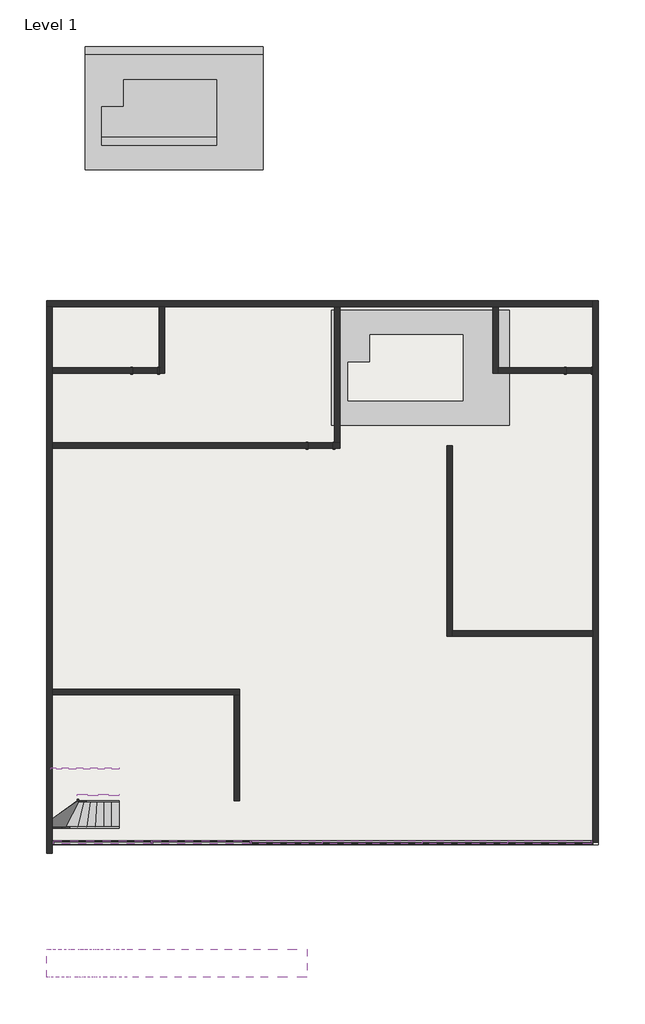
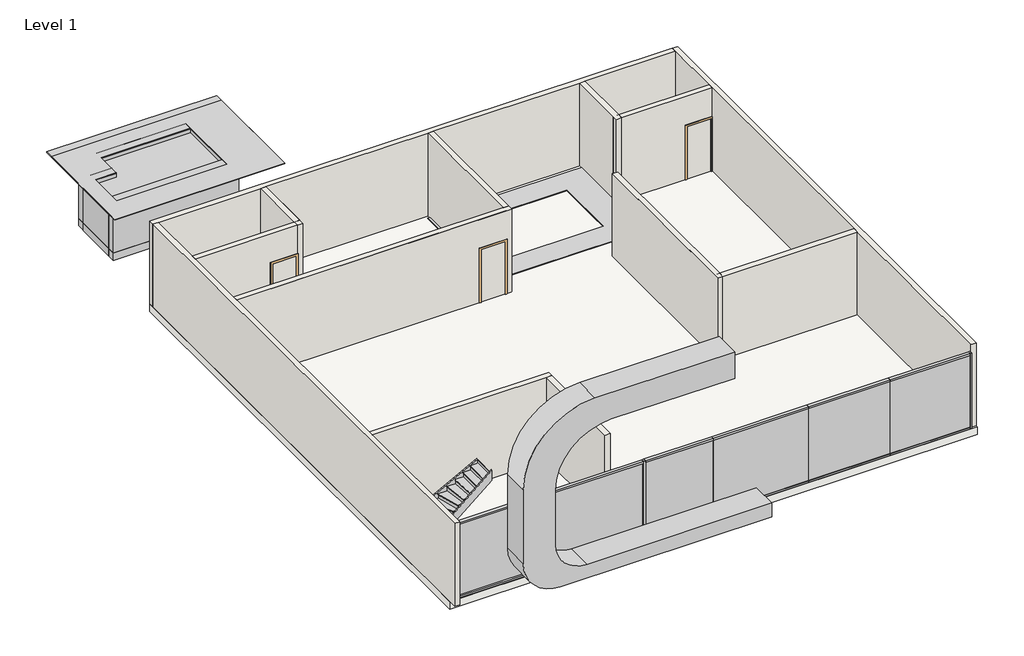
# One storey, incomplete: 32 members, 26 walls, 6 plates, 3 doors, 3 furniture elements, 2 slabs, 2 stair flights, 1 proxy.
"""IFC4 building model written with IfcOpenShell, lengths in millimetres."""

from ifc_helpers import new_model, si_unit, frame, origin, origin_with_axes, place, context, project, spatial, polyline, outline, extrude, faceted_brep, transform, mapped, element, save
from components import generic_models_1_generic_models_1_6508f6ba, door_54dd4da4, door_719f80de, swimming_pool_w_adjustable_terrace_and_size_parametric_16462_e4165495, member_3f395ae9, member_901dee17, member_eaba9652, member_a37e84cf, member_e3dca2c5, member_9f3fc137, member_47c71a51, system_panel_glazed_4ffbc40e, system_panel_glazed_c3829408, system_panel_glazed_34d630f4, system_panel_glazed_dc472efa, system_panel_glazed_7998c3ce, stair_flight_c9f3f3be

model = new_model("IFC4")

# Units and contexts
model_context = context("Model", 3, world=origin())
ifc_project = project(units=[si_unit("LENGTHUNIT", "METRE", prefix="MILLI")], contexts=[model_context])

# Site, building, storey
site = spatial("IfcSite", under=ifc_project)
building = spatial("IfcBuilding", under=site)
storey = spatial("IfcBuildingStorey", under=building, Name="Level 1", Elevation=0.0)

# Proxy
placement = place(None, origin())
generic_models_1_generic_models_1_shape = generic_models_1_generic_models_1_6508f6ba(model_context)
element("IfcBuildingElementProxy", 1, Name="Generic Models 1 : Generic Models 1", ObjectType="Generic Models 1 : Generic Models 1", at=placement, inside=storey, context=model_context, shape_type="MappedRepresentation", body=[
    mapped(generic_models_1_generic_models_1_shape, transform((0.0, 0.0, 0.0), x_axis=(1.0, 0.0, 0.0), y_axis=(0.0, 1.0, 0.0), z_axis=(0.0, 0.0, 1.0))),
])

# Doors
door_shape = door_54dd4da4(model_context)
element("IfcDoor", 2, ObjectType="Single-Flush : 36\" x 84\"", at=placement, inside=storey, context=model_context, shape_type="MappedRepresentation", body=[
    mapped(door_shape, transform((-345.7931824, 3798.689221, 0.0), x_axis=(1.0, 0.0, 0.0), y_axis=(0.0, 1.0, 0.0), z_axis=(0.0, 0.0, 1.0))),
])
element("IfcDoor", 3, ObjectType="Single-Flush : 36\" x 84\"", at=placement, inside=storey, context=model_context, shape_type="MappedRepresentation", body=[
    mapped(door_shape, transform((-6746.5931824, 6541.889221, 0.0), x_axis=(1.0, 0.0, 0.0), y_axis=(0.0, 1.0, 0.0), z_axis=(0.0, 0.0, 1.0))),
])
door_2_shape = door_719f80de(model_context)
element("IfcDoor", 4, ObjectType="Single-Flush : 36\" x 84\"", at=placement, inside=storey, context=model_context, shape_type="MappedRepresentation", body=[
    mapped(door_2_shape, transform((9103.0068176, 6541.889221, 0.0), x_axis=(-1.0, 0.0, 0.0), y_axis=(0.0, -1.0, 0.0), z_axis=(0.0, 0.0, 1.0))),
])

# Furniture
swimming_pool_w_adjustable_terrace_and_size_parametric_16462_shape = swimming_pool_w_adjustable_terrace_and_size_parametric_16462_e4165495(model_context)
element("IfcFurniture", 5, ObjectType="Swimming_pool_w_adjustable_terrace_and_size_parametric_16462 : Swimming_pool_w_adjustable_terrace_and_size_parametric_16462", at=placement, inside=storey, context=model_context, shape_type="MappedRepresentation", body=[
    mapped(swimming_pool_w_adjustable_terrace_and_size_parametric_16462_shape, transform((-6238.5931824, 15966.689221, 0.0), x_axis=(1.0, 0.0, 0.0), y_axis=(0.0, 1.0, 0.0), z_axis=(0.0, 0.0, 1.0))),
])
element("IfcFurniture", 6, ObjectType="Swimming_pool_w_adjustable_terrace_and_size_parametric_16462 : Swimming_pool_w_adjustable_terrace_and_size_parametric_16462", at=placement, inside=storey, context=model_context, shape_type="MappedRepresentation", body=[
    mapped(swimming_pool_w_adjustable_terrace_and_size_parametric_16462_shape, transform((-6238.5931824, 16271.489221, 0.0), x_axis=(1.0, 0.0, 0.0), y_axis=(0.0, 1.0, 0.0), z_axis=(0.0, 0.0, 1.0))),
])
element("IfcFurniture", 7, ObjectType="Swimming_pool_w_adjustable_terrace_and_size_parametric_16462 : Swimming_pool_w_adjustable_terrace_and_size_parametric_16462", at=placement, inside=storey, context=model_context, shape_type="MappedRepresentation", body=[
    mapped(swimming_pool_w_adjustable_terrace_and_size_parametric_16462_shape, transform((2765.4068176, 6643.489221, 0.0), x_axis=(1.0, 0.0, 0.0), y_axis=(0.0, 1.0, 0.0), z_axis=(0.0, 0.0, 1.0))),
])

# Members
member_shape = member_3f395ae9(model_context)
element("IfcMember", 8, ObjectType="Rectangular Mullion : 2.5\" x 5\" rectangular", at=placement, inside=storey, context=model_context, shape_type="MappedRepresentation", body=[
    mapped(member_shape, transform((-2854.6898891, -10679.310779, 0.0), x_axis=(1.0, 0.0, 0.0), y_axis=(0.0, -1.0, 0.0), z_axis=(0.0, 0.0, -1.0))),
])
element("IfcMember", 9, ObjectType="Rectangular Mullion : 2.5\" x 5\" rectangular", at=placement, inside=storey, context=model_context, shape_type="MappedRepresentation", body=[
    mapped(member_shape, transform((-10150.1931824, -10679.310779, 3048.0), x_axis=(-1.0, 0.0, 0.0), y_axis=(0.0, -1.0, 0.0), z_axis=(0.0, 0.0, 1.0))),
])
element("IfcMember", 10, ObjectType="Rectangular Mullion : 2.5\" x 5\" rectangular", at=placement, inside=storey, context=model_context, shape_type="MappedRepresentation", body=[
    mapped(member_shape, transform((9611.0068176, -10679.310779, 3048.0), x_axis=(1.0, 0.0, 0.0), y_axis=(0.0, 1.0, 0.0), z_axis=(0.0, 0.0, 1.0))),
])
member_2_shape = member_901dee17(model_context)
element("IfcMember", 11, ObjectType="Rectangular Mullion : 2.5\" x 5\" rectangular", at=placement, inside=storey, context=model_context, shape_type="MappedRepresentation", body=[
    mapped(member_2_shape, transform((-10086.6931824, -10679.310779, 0.0), x_axis=(0.0, 0.0, -1.0), y_axis=(0.0, -1.0, 0.0), z_axis=(-1.0, 0.0, 0.0))),
])
element("IfcMember", 12, ObjectType="Rectangular Mullion : 2.5\" x 5\" rectangular", at=placement, inside=storey, context=model_context, shape_type="MappedRepresentation", body=[
    mapped(member_2_shape, transform((-6470.6915358, -10679.310779, 0.0), x_axis=(0.0, 0.0, -1.0), y_axis=(0.0, -1.0, 0.0), z_axis=(-1.0, 0.0, 0.0))),
])
element("IfcMember", 13, ObjectType="Rectangular Mullion : 2.5\" x 5\" rectangular", at=placement, inside=storey, context=model_context, shape_type="MappedRepresentation", body=[
    mapped(member_2_shape, transform((-2918.1898891, -10679.310779, 3048.0), x_axis=(0.0, 0.0, 1.0), y_axis=(0.0, -1.0, 0.0), z_axis=(1.0, 0.0, 0.0))),
])
element("IfcMember", 14, ObjectType="Rectangular Mullion : 2.5\" x 5\" rectangular", at=placement, inside=storey, context=model_context, shape_type="MappedRepresentation", body=[
    mapped(member_2_shape, transform((-6534.1915358, -10679.310779, 3048.0), x_axis=(0.0, 0.0, 1.0), y_axis=(0.0, -1.0, 0.0), z_axis=(1.0, 0.0, 0.0))),
])
member_3_shape = member_eaba9652(model_context)
element("IfcMember", 15, ObjectType="Rectangular Mullion : 2.5\" x 5\" rectangular", at=placement, inside=storey, context=model_context, shape_type="MappedRepresentation", body=[
    mapped(member_3_shape, transform((-6502.4415358, -10679.310779, 0.0), x_axis=(1.0, 0.0, 0.0), y_axis=(0.0, -1.0, 0.0), z_axis=(0.0, 0.0, -1.0))),
])
member_4_shape = member_a37e84cf(model_context)
element("IfcMember", 16, ObjectType="Rectangular Mullion : 2.5\" x 5\" rectangular", at=placement, inside=storey, context=model_context, shape_type="MappedRepresentation", body=[
    mapped(member_4_shape, transform((9547.5068176, -10679.310779, 0.0), x_axis=(0.0, 0.0, -1.0), y_axis=(0.0, 1.0, 0.0), z_axis=(1.0, 0.0, 0.0))),
])
member_5_shape = member_e3dca2c5(model_context)
element("IfcMember", 17, ObjectType="Rectangular Mullion : 2.5\" x 5\" rectangular", at=placement, inside=storey, context=model_context, shape_type="MappedRepresentation", body=[
    mapped(member_5_shape, transform((3378.1584642, -10679.310779, 3048.0), x_axis=(0.0, 0.0, 1.0), y_axis=(0.0, 1.0, 0.0), z_axis=(-1.0, 0.0, 0.0))),
])
element("IfcMember", 18, ObjectType="Rectangular Mullion : 2.5\" x 5\" rectangular", at=placement, inside=storey, context=model_context, shape_type="MappedRepresentation", body=[
    mapped(member_5_shape, transform((6494.5826409, -10679.310779, 0.0), x_axis=(0.0, 0.0, -1.0), y_axis=(0.0, 1.0, 0.0), z_axis=(1.0, 0.0, 0.0))),
])
element("IfcMember", 19, ObjectType="Rectangular Mullion : 2.5\" x 5\" rectangular", at=placement, inside=storey, context=model_context, shape_type="MappedRepresentation", body=[
    mapped(member_4_shape, transform((6494.5826409, -10679.310779, 3048.0), x_axis=(0.0, 0.0, 1.0), y_axis=(0.0, 1.0, 0.0), z_axis=(-1.0, 0.0, 0.0))),
])
member_6_shape = member_9f3fc137(model_context)
element("IfcMember", 20, ObjectType="Rectangular Mullion : 2.5\" x 5\" rectangular", at=placement, inside=storey, context=model_context, shape_type="MappedRepresentation", body=[
    mapped(member_6_shape, transform((-2854.6898891, -10679.310779, 3048.0), x_axis=(0.0, 0.0, 1.0), y_axis=(0.0, 1.0, 0.0), z_axis=(-1.0, 0.0, 0.0))),
])
member_7_shape = member_47c71a51(model_context)
element("IfcMember", 21, ObjectType="Rectangular Mullion : 2.5\" x 5\" rectangular", at=placement, inside=storey, context=model_context, shape_type="MappedRepresentation", body=[
    mapped(member_7_shape, transform((3378.1584642, -10679.310779, 0.0), x_axis=(0.0, 0.0, -1.0), y_axis=(0.0, 1.0, 0.0), z_axis=(1.0, 0.0, 0.0))),
])
element("IfcMember", 22, ObjectType="Rectangular Mullion : 2.5\" x 5\" rectangular", at=placement, inside=storey, context=model_context, shape_type="MappedRepresentation", body=[
    mapped(member_7_shape, transform((-263.8898891, -10679.310779, 3048.0), x_axis=(0.0, 0.0, 1.0), y_axis=(0.0, 1.0, 0.0), z_axis=(-1.0, 0.0, 0.0))),
])
element("IfcMember", 23, ObjectType="Rectangular Mullion : 2.5\" x 5\" rectangular", at=placement, inside=storey, context=model_context, shape_type="MappedRepresentation", body=[
    mapped(member_6_shape, transform((-263.8898891, -10679.310779, 0.0), x_axis=(0.0, 0.0, -1.0), y_axis=(0.0, 1.0, 0.0), z_axis=(1.0, 0.0, 0.0))),
])
element("IfcMember", 24, ObjectType="Stringer - 2\" Width", at=placement, inside=storey, context=model_context, shape_type="SweptSolid", body=[
    extrude(outline(polyline([(0.0, -7708.0614906), (232.4562572, -7708.0614906), (1353.5069249, -9795.4786823), (1007.5321542, -9795.4786823), (0.0, -7919.4350738), (0.0, -7708.0614906)])), frame((0.0, -10171.310779, 0.0), z_axis=(0.0, 1.0, 0.0), x_axis=(0.0, 0.0, 1.0)), (0.0, 0.0, 1.0), 50.8),
])
element("IfcMember", 25, ObjectType="Stringer - 2\" Width", at=placement, inside=storey, context=model_context, shape_type="SweptSolid", body=[
    extrude(outline(polyline([(-9795.4786823, -10120.510779), (-9795.4786823, -10171.310779), (-10150.1931824, -10171.310779), (-10150.1931824, -10120.510779), (-9795.4786823, -10120.510779)])), frame((0.0, 0.0, 1007.5321542), z_axis=(0.0, 0.0, 1.0), x_axis=(1.0, 0.0, 0.0)), (0.0, 0.0, 1.0), 345.9747707),
])
element("IfcMember", 26, ObjectType="Stringer - 2\" Width", at=placement, inside=storey, context=model_context, shape_type="SweptSolid", body=[
    extrude(outline(polyline([(-10171.310779, 1048.7069249), (-10171.310779, 1336.5201671), (-8051.2752516, 2045.4282369), (-8012.310779, 2045.4282369), (-8012.310779, 1712.4826013), (-9997.3749587, 1048.7069249), (-10171.310779, 1048.7069249)])), frame((-10200.9931824, 0.0, 0.0), z_axis=(1.0, 0.0, 0.0), x_axis=(0.0, 1.0, 0.0)), (0.0, 0.0, 1.0), 50.8),
])
element("IfcMember", 27, ObjectType="Stringer - 2\" Width", at=placement, inside=storey, context=model_context, shape_type="SweptSolid", body=[
    extrude(outline(polyline([(-10200.9931824, -8012.310779), (-10200.9931824, -7961.510779), (-9795.4786823, -7961.510779), (-9795.4786823, -8012.310779), (-10200.9931824, -8012.310779)])), frame((0.0, 0.0, 1724.0393171), z_axis=(0.0, 0.0, 1.0), x_axis=(1.0, 0.0, 0.0)), (0.0, 0.0, 1.0), 321.3889199),
])
element("IfcMember", 28, ObjectType="Stringer - 2\" Width", at=placement, inside=storey, context=model_context, shape_type="SweptSolid", body=[
    extrude(outline(polyline([(2045.4282369, -9795.4786823), (1724.0393171, -9795.4786823), (2845.0899847, -7708.0614906), (3166.4789046, -7708.0614906), (2045.4282369, -9795.4786823)])), frame((0.0, -8012.310779, 0.0), z_axis=(0.0, 1.0, 0.0), x_axis=(0.0, 0.0, 1.0)), (0.0, 0.0, 1.0), 50.8),
])
element("IfcMember", 29, ObjectType="Stringer - 2\" Width", at=placement, inside=storey, context=model_context, shape_type="SweptSolid", body=[
    extrude(outline(polyline([(0.0, -7708.0614906), (177.9241916, -7708.0614906), (1432.8713283, -9184.9931824), (1032.8989166, -9184.9931824), (0.0, -7969.3872818), (0.0, -7708.0614906)])), frame((0.0, -9206.110779, 0.0), z_axis=(0.0, 1.0, 0.0), x_axis=(0.0, 0.0, 1.0)), (0.0, 0.0, 1.0), 50.8),
])
element("IfcMember", 30, ObjectType="Stringer - 2\" Width", at=placement, inside=storey, context=model_context, shape_type="SweptSolid", body=[
    extrude(outline(polyline([(-9206.110779, 1076.0636174), (-9206.110779, 1636.5940989), (-9001.0207186, 2001.5714311), (-8977.510779, 2001.5714311), (-8977.510779, 1421.2173278), (-9171.4614414, 1076.0636174), (-9206.110779, 1076.0636174)])), frame((-9235.7931824, 0.0, 0.0), z_axis=(1.0, 0.0, 0.0), x_axis=(0.0, 1.0, 0.0)), (0.0, 0.0, 1.0), 50.8),
])
element("IfcMember", 31, ObjectType="Stringer - 2\" Width", at=placement, inside=storey, context=model_context, shape_type="SweptSolid", body=[
    extrude(outline(polyline([(2001.5714311, -9235.7931824), (1601.5990193, -9235.7931824), (2899.7108568, -7708.0614906), (3299.6832686, -7708.0614906), (2001.5714311, -9235.7931824)])), frame((0.0, -8977.510779, 0.0), z_axis=(0.0, 1.0, 0.0), x_axis=(0.0, 0.0, 1.0)), (0.0, 0.0, 1.0), 50.8),
])
element("IfcMember", 32, ObjectType="Stringer - 2\" Width", at=placement, inside=storey, context=model_context, shape_type="SweptSolid", body=[
    extrude(outline(polyline([(0.0, -7708.0614906), (232.4562572, -7708.0614906), (1353.5069249, -9795.4786823), (1007.5321542, -9795.4786823), (0.0, -7919.4350738), (0.0, -7708.0614906)])), frame((0.0, -10171.310779, 0.0), z_axis=(0.0, 1.0, 0.0), x_axis=(0.0, 0.0, 1.0)), (0.0, 0.0, 1.0), 50.8),
])
element("IfcMember", 33, ObjectType="Stringer - 2\" Width", at=placement, inside=storey, context=model_context, shape_type="SweptSolid", body=[
    extrude(outline(polyline([(-9795.4786823, -10120.510779), (-9795.4786823, -10171.310779), (-10150.1931824, -10171.310779), (-10150.1931824, -10120.510779), (-9795.4786823, -10120.510779)])), frame((0.0, 0.0, 1007.5321542), z_axis=(0.0, 0.0, 1.0), x_axis=(1.0, 0.0, 0.0)), (0.0, 0.0, 1.0), 345.9747707),
])
element("IfcMember", 34, ObjectType="Stringer - 2\" Width", at=placement, inside=storey, context=model_context, shape_type="SweptSolid", body=[
    extrude(outline(polyline([(-10171.310779, 1048.7069249), (-10171.310779, 1336.5201671), (-8051.2752516, 2045.4282369), (-8012.310779, 2045.4282369), (-8012.310779, 1712.4826013), (-9997.3749587, 1048.7069249), (-10171.310779, 1048.7069249)])), frame((-10200.9931824, 0.0, 0.0), z_axis=(1.0, 0.0, 0.0), x_axis=(0.0, 1.0, 0.0)), (0.0, 0.0, 1.0), 50.8),
])
element("IfcMember", 35, ObjectType="Stringer - 2\" Width", at=placement, inside=storey, context=model_context, shape_type="SweptSolid", body=[
    extrude(outline(polyline([(-10200.9931824, -8012.310779), (-10200.9931824, -7961.510779), (-9795.4786823, -7961.510779), (-9795.4786823, -8012.310779), (-10200.9931824, -8012.310779)])), frame((0.0, 0.0, 1724.0393171), z_axis=(0.0, 0.0, 1.0), x_axis=(1.0, 0.0, 0.0)), (0.0, 0.0, 1.0), 321.3889199),
])
element("IfcMember", 36, ObjectType="Stringer - 2\" Width", at=placement, inside=storey, context=model_context, shape_type="SweptSolid", body=[
    extrude(outline(polyline([(2045.4282369, -9795.4786823), (1724.0393171, -9795.4786823), (2845.0899847, -7708.0614906), (3166.4789046, -7708.0614906), (2045.4282369, -9795.4786823)])), frame((0.0, -8012.310779, 0.0), z_axis=(0.0, 1.0, 0.0), x_axis=(0.0, 0.0, 1.0)), (0.0, 0.0, 1.0), 50.8),
])
element("IfcMember", 37, ObjectType="Stringer - 2\" Width", at=placement, inside=storey, context=model_context, shape_type="SweptSolid", body=[
    extrude(outline(polyline([(0.0, -7708.0614906), (177.9241916, -7708.0614906), (1432.8713283, -9184.9931824), (1032.8989166, -9184.9931824), (0.0, -7969.3872818), (0.0, -7708.0614906)])), frame((0.0, -9206.110779, 0.0), z_axis=(0.0, 1.0, 0.0), x_axis=(0.0, 0.0, 1.0)), (0.0, 0.0, 1.0), 50.8),
])
element("IfcMember", 38, ObjectType="Stringer - 2\" Width", at=placement, inside=storey, context=model_context, shape_type="SweptSolid", body=[
    extrude(outline(polyline([(-9206.110779, 1076.0636174), (-9206.110779, 1636.5940989), (-9001.0207186, 2001.5714311), (-8977.510779, 2001.5714311), (-8977.510779, 1421.2173278), (-9171.4614414, 1076.0636174), (-9206.110779, 1076.0636174)])), frame((-9235.7931824, 0.0, 0.0), z_axis=(1.0, 0.0, 0.0), x_axis=(0.0, 1.0, 0.0)), (0.0, 0.0, 1.0), 50.8),
])
element("IfcMember", 39, ObjectType="Stringer - 2\" Width", at=placement, inside=storey, context=model_context, shape_type="SweptSolid", body=[
    extrude(outline(polyline([(2001.5714311, -9235.7931824), (1601.5990193, -9235.7931824), (2899.7108568, -7708.0614906), (3299.6832686, -7708.0614906), (2001.5714311, -9235.7931824)])), frame((0.0, -8977.510779, 0.0), z_axis=(0.0, 1.0, 0.0), x_axis=(0.0, 0.0, 1.0)), (0.0, 0.0, 1.0), 50.8),
])

# Plates
system_panel_glazed_shape = system_panel_glazed_4ffbc40e(model_context)
element("IfcPlate", 40, ObjectType="System Panel : Glazed", at=placement, inside=storey, context=model_context, shape_type="MappedRepresentation", body=[
    mapped(system_panel_glazed_shape, transform((-8310.4423591, -10679.310779, 63.5), x_axis=(1.0, 0.0, 0.0), y_axis=(0.0, 1.0, 0.0), z_axis=(0.0, 0.0, 1.0))),
])
element("IfcPlate", 41, ObjectType="System Panel : Glazed", at=placement, inside=storey, context=model_context, shape_type="MappedRepresentation", body=[
    mapped(system_panel_glazed_shape, transform((-4694.4407124, -10679.310779, 63.5), x_axis=(1.0, 0.0, 0.0), y_axis=(0.0, 1.0, 0.0), z_axis=(0.0, 0.0, 1.0))),
])
system_panel_glazed_2_shape = system_panel_glazed_c3829408(model_context)
element("IfcPlate", 42, ObjectType="System Panel : Glazed", at=placement, inside=storey, context=model_context, shape_type="MappedRepresentation", body=[
    mapped(system_panel_glazed_2_shape, transform((8021.0447292, -10679.310779, 63.5), x_axis=(-1.0, 0.0, 0.0), y_axis=(0.0, -1.0, 0.0), z_axis=(0.0, 0.0, 1.0))),
])
system_panel_glazed_3_shape = system_panel_glazed_34d630f4(model_context)
element("IfcPlate", 43, ObjectType="System Panel : Glazed", at=placement, inside=storey, context=model_context, shape_type="MappedRepresentation", body=[
    mapped(system_panel_glazed_3_shape, transform((4936.3705526, -10679.310779, 63.5), x_axis=(-1.0, 0.0, 0.0), y_axis=(0.0, -1.0, 0.0), z_axis=(0.0, 0.0, 1.0))),
])
system_panel_glazed_4_shape = system_panel_glazed_dc472efa(model_context)
element("IfcPlate", 44, ObjectType="System Panel : Glazed", at=placement, inside=storey, context=model_context, shape_type="MappedRepresentation", body=[
    mapped(system_panel_glazed_4_shape, transform((1557.1342876, -10679.310779, 63.5), x_axis=(-1.0, 0.0, 0.0), y_axis=(0.0, -1.0, 0.0), z_axis=(0.0, 0.0, 1.0))),
])
system_panel_glazed_5_shape = system_panel_glazed_7998c3ce(model_context)
element("IfcPlate", 45, ObjectType="System Panel : Glazed", at=placement, inside=storey, context=model_context, shape_type="MappedRepresentation", body=[
    mapped(system_panel_glazed_5_shape, transform((-1559.2898891, -10679.310779, 63.5), x_axis=(-1.0, 0.0, 0.0), y_axis=(0.0, -1.0, 0.0), z_axis=(0.0, 0.0, 1.0))),
])

# Slabs
element("IfcSlab", 46, ObjectType="Generic - 12\"", at=placement, inside=storey, context=model_context, shape_type="SweptSolid", body=[
    extrude(outline(polyline([(-10353.3931824, -10769.1988659), (-10353.3931824, 9081.889221), (9814.2068176, 9081.889221), (9814.2068176, -10769.1988659), (-10353.3931824, -10769.1988659)])), frame((0.0, 0.0, -304.8), z_axis=(0.0, 0.0, 1.0), x_axis=(1.0, 0.0, 0.0)), (0.0, 0.0, 1.0), 304.8),
])
element("IfcSlab", 47, ObjectType="Generic - 12\"", at=placement, inside=storey, context=model_context, shape_type="SweptSolid", body=[
    extrude(outline(polyline([(-10353.3931824, -10769.1988659), (-10353.3931824, 9081.889221), (9814.2068176, 9081.889221), (9814.2068176, -10769.1988659), (-10353.3931824, -10769.1988659)])), frame((0.0, 0.0, -304.8), z_axis=(0.0, 0.0, 1.0), x_axis=(1.0, 0.0, 0.0)), (0.0, 0.0, 1.0), 304.8),
])

# Stair flights
stair_flight_shape = stair_flight_c9f3f3be(model_context)
element("IfcStairFlight", 48, ObjectType="2\" Tread 1\" Nosing 1/4\" Riser", at=placement, inside=storey, context=model_context, shape_type="MappedRepresentation", body=[
    mapped(stair_flight_shape, transform((0.0, 0.0, 0.0), x_axis=(1.0, 0.0, 0.0), y_axis=(0.0, 1.0, 0.0), z_axis=(0.0, 0.0, 1.0))),
])
element("IfcStairFlight", 49, ObjectType="2\" Tread 1\" Nosing 1/4\" Riser", at=placement, inside=storey, context=model_context, shape_type="MappedRepresentation", body=[
    mapped(stair_flight_shape, transform((0.0, 0.0, 0.0), x_axis=(1.0, 0.0, 0.0), y_axis=(0.0, 1.0, 0.0), z_axis=(0.0, 0.0, 1.0))),
])

# Walls
element("IfcWall", 50, ObjectType="wall.1", at=placement, inside=storey, context=model_context, shape_type="Brep", body=[
    faceted_brep([(-10353.3931824, 8878.689221, 0.0), (-10150.1931824, 8878.689221, 0.0), (-6238.5931824, 8878.689221, 0.0), (-6035.3931824, 8878.689221, 0.0), (162.2068176, 8878.689221, 0.0), (365.4068176, 8878.689221, 0.0), (5953.4068176, 8878.689221, 0.0), (6156.6068176, 8878.689221, 0.0), (9611.0068176, 8878.689221, 0.0), (9611.0068176, 8878.689221, 3352.8), (6156.6068176, 8878.689221, 3352.8), (5953.4068176, 8878.689221, 3352.8), (365.4068176, 8878.689221, 3352.8), (162.2068176, 8878.689221, 3352.8), (-6035.3931824, 8878.689221, 3352.8), (-6238.5931824, 8878.689221, 3352.8), (-10150.1931824, 8878.689221, 3352.8), (-10353.3931824, 8878.689221, 3352.8), (-10353.3931824, 9081.889221, 0.0), (-10353.3931824, 9081.889221, 3352.8), (9611.0068176, 9081.889221, 3352.8), (9611.0068176, 9081.889221, 0.0)], [[[0, 1, 2, 3, 4, 5, 6, 7, 8, 9, 10, 11, 12, 13, 14, 15, 16, 17]], [[18, 19, 20, 21]], [[8, 7, 6, 5, 4, 3, 2, 1, 0, 18, 21]], [[17, 16, 15, 14, 13, 12, 11, 10, 9, 20, 19]], [[0, 17, 19, 18]], [[9, 8, 21, 20]]]),
])
element("IfcWall", 51, ObjectType="wall.1", at=placement, inside=storey, context=model_context, shape_type="Brep", body=[
    faceted_brep([(-10150.1931824, -11085.710779, 0.0), (-10150.1931824, -5294.510779, 0.0), (-10150.1931824, -5091.310779, 0.0), (-10150.1931824, 3697.089221, 0.0), (-10150.1931824, 3900.289221, 0.0), (-10150.1931824, 6440.289221, 0.0), (-10150.1931824, 6643.489221, 0.0), (-10150.1931824, 8878.689221, 0.0), (-10150.1931824, 8878.689221, 3352.8), (-10150.1931824, 6643.489221, 3352.8), (-10150.1931824, 6440.289221, 3352.8), (-10150.1931824, 3900.289221, 3352.8), (-10150.1931824, 3697.089221, 3352.8), (-10150.1931824, -5091.310779, 3352.8), (-10150.1931824, -5294.510779, 3352.8), (-10150.1931824, -11085.710779, 3352.8), (-10353.3931824, -11085.710779, 0.0), (-10353.3931824, -11085.710779, 3352.8), (-10353.3931824, 8878.689221, 3352.8), (-10353.3931824, 8878.689221, 0.0)], [[[0, 1, 2, 3, 4, 5, 6, 7, 8, 9, 10, 11, 12, 13, 14, 15]], [[16, 17, 18, 19]], [[7, 6, 5, 4, 3, 2, 1, 0, 16, 19]], [[15, 14, 13, 12, 11, 10, 9, 8, 18, 17]], [[0, 15, 17, 16]], [[8, 7, 19, 18]]]),
])
element("IfcWall", 52, ObjectType="wall.1", at=placement, inside=storey, context=model_context, shape_type="Brep", body=[
    faceted_brep([(9611.0068176, 9081.889221, 0.0), (9611.0068176, 8878.689221, 0.0), (9611.0068176, 6643.489221, 0.0), (9611.0068176, 6440.289221, 0.0), (9611.0068176, -2957.710779, 0.0), (9611.0068176, -3160.910779, 0.0), (9611.0068176, -10679.310779, 0.0), (9611.0068176, -10679.310779, 3352.8), (9611.0068176, -3160.910779, 3352.8), (9611.0068176, -2957.710779, 3352.8), (9611.0068176, 6440.289221, 3352.8), (9611.0068176, 6643.489221, 3352.8), (9611.0068176, 8878.689221, 3352.8), (9611.0068176, 9081.889221, 3352.8), (9814.2068176, 9081.889221, 0.0), (9814.2068176, 9081.889221, 3352.8), (9814.2068176, -10679.310779, 3352.8), (9814.2068176, -10679.310779, 0.0)], [[[0, 1, 2, 3, 4, 5, 6, 7, 8, 9, 10, 11, 12, 13]], [[14, 15, 16, 17]], [[6, 5, 4, 3, 2, 1, 0, 14, 17]], [[7, 6, 17, 16]], [[13, 12, 11, 10, 9, 8, 7, 16, 15]], [[0, 13, 15, 14]]]),
])
element("IfcWall", 53, ObjectType="wall.1", at=placement, inside=storey, context=model_context, shape_type="SweptSolid", body=[
    extrude(outline(polyline([(162.2068176, 3900.289221), (162.2068176, 8878.689221), (365.4068176, 8878.689221), (365.4068176, 3900.289221), (162.2068176, 3900.289221)])), origin_with_axes(), (0.0, 0.0, 1.0), 3352.8),
])
element("IfcWall", 54, ObjectType="wall.1", at=placement, inside=storey, context=model_context, shape_type="Brep", body=[
    faceted_brep([(365.4068176, 3900.289221, 0.0), (162.2068176, 3900.289221, 0.0), (111.4068176, 3900.289221, 0.0), (111.4068176, 3900.289221, 2133.6), (-802.9931824, 3900.289221, 2133.6), (-802.9931824, 3900.289221, 0.0), (-10150.1931824, 3900.289221, 0.0), (-10150.1931824, 3900.289221, 3352.8), (162.2068176, 3900.289221, 3352.8), (365.4068176, 3900.289221, 3352.8), (111.4068176, 3697.089221, 2133.6), (111.4068176, 3697.089221, 0.0), (365.4068176, 3697.089221, 0.0), (365.4068176, 3697.089221, 3352.8), (-10150.1931824, 3697.089221, 3352.8), (-10150.1931824, 3697.089221, 0.0), (-802.9931824, 3697.089221, 0.0), (-802.9931824, 3697.089221, 2133.6)], [[[0, 1, 2, 3, 4, 5, 6, 7, 8, 9]], [[10, 11, 12, 13, 14, 15, 16, 17]], [[16, 15, 6, 5]], [[12, 11, 2, 1, 0]], [[9, 8, 7, 14, 13]], [[7, 6, 15, 14]], [[0, 9, 13, 12]], [[3, 2, 11, 10]], [[4, 3, 10, 17]], [[5, 4, 17, 16]]]),
])
element("IfcWall", 55, ObjectType="wall.1", at=placement, inside=storey, context=model_context, shape_type="Brep", body=[
    faceted_brep([(-6238.5931824, 8878.689221, 0.0), (-6238.5931824, 6643.489221, 0.0), (-6238.5931824, 6440.289221, 0.0), (-6238.5931824, 6440.289221, 3352.8), (-6238.5931824, 6643.489221, 3352.8), (-6238.5931824, 8878.689221, 3352.8), (-6035.3931824, 8878.689221, 0.0), (-6035.3931824, 8878.689221, 3352.8), (-6035.3931824, 6440.289221, 3352.8), (-6035.3931824, 6440.289221, 0.0)], [[[0, 1, 2, 3, 4, 5]], [[6, 7, 8, 9]], [[2, 1, 0, 6, 9]], [[5, 4, 3, 8, 7]], [[0, 5, 7, 6]], [[3, 2, 9, 8]]]),
])
element("IfcWall", 56, ObjectType="wall.1", at=placement, inside=storey, context=model_context, shape_type="SweptSolid", body=[
    extrude(outline(polyline([(2133.6, -6289.3931824), (0.0, -6289.3931824), (0.0, -6238.5931824), (3352.8, -6238.5931824), (3352.8, -10150.1931824), (0.0, -10150.1931824), (0.0, -7203.7931824), (2133.6, -7203.7931824), (2133.6, -6289.3931824)])), frame((0.0, 6440.289221, 0.0), z_axis=(0.0, 1.0, 0.0), x_axis=(0.0, 0.0, 1.0)), (0.0, 0.0, 1.0), 203.2),
])
element("IfcWall", 57, ObjectType="wall.1", at=placement, inside=storey, context=model_context, shape_type="Brep", body=[
    faceted_brep([(5953.4068176, 8878.689221, 0.0), (5953.4068176, 6440.289221, 0.0), (5953.4068176, 6440.289221, 3352.8), (5953.4068176, 8878.689221, 3352.8), (6156.6068176, 8878.689221, 0.0), (6156.6068176, 8878.689221, 3352.8), (6156.6068176, 6643.489221, 3352.8), (6156.6068176, 6440.289221, 3352.8), (6156.6068176, 6440.289221, 0.0), (6156.6068176, 6643.489221, 0.0)], [[[0, 1, 2, 3]], [[4, 5, 6, 7, 8, 9]], [[1, 0, 4, 9, 8]], [[3, 2, 7, 6, 5]], [[0, 3, 5, 4]], [[2, 1, 8, 7]]]),
])
element("IfcWall", 58, ObjectType="wall.1", at=placement, inside=storey, context=model_context, shape_type="SweptSolid", body=[
    extrude(outline(polyline([(0.0, 6156.6068176), (0.0, 8645.8068176), (2133.6, 8645.8068176), (2133.6, 9560.2068176), (0.0, 9560.2068176), (0.0, 9611.0068176), (3352.8, 9611.0068176), (3352.8, 6156.6068176), (0.0, 6156.6068176)])), frame((0.0, 6440.289221, 0.0), z_axis=(0.0, 1.0, 0.0), x_axis=(0.0, 0.0, 1.0)), (0.0, 0.0, 1.0), 203.2),
])
element("IfcWall", 59, ObjectType="wall.1", at=placement, inside=storey, context=model_context, shape_type="Brep", body=[
    faceted_brep([(4277.0068176, 3798.689221, 0.0), (4277.0068176, -3160.910779, 0.0), (4277.0068176, -3160.910779, 3352.8), (4277.0068176, 3798.689221, 3352.8), (4480.2068176, 3798.689221, 0.0), (4480.2068176, 3798.689221, 3352.8), (4480.2068176, -2957.710779, 3352.8), (4480.2068176, -3160.910779, 3352.8), (4480.2068176, -3160.910779, 0.0), (4480.2068176, -2957.710779, 0.0)], [[[0, 1, 2, 3]], [[4, 5, 6, 7, 8, 9]], [[1, 0, 4, 9, 8]], [[3, 2, 7, 6, 5]], [[0, 3, 5, 4]], [[2, 1, 8, 7]]]),
])
element("IfcWall", 60, ObjectType="wall.1", at=placement, inside=storey, context=model_context, shape_type="SweptSolid", body=[
    extrude(outline(polyline([(9611.0068176, -3160.910779), (4480.2068176, -3160.910779), (4480.2068176, -2957.710779), (9611.0068176, -2957.710779), (9611.0068176, -3160.910779)])), origin_with_axes(), (0.0, 0.0, 1.0), 3352.8),
])
element("IfcWall", 61, ObjectType="wall.1", at=placement, inside=storey, context=model_context, shape_type="Brep", body=[
    faceted_brep([(-10150.1931824, -5294.510779, 0.0), (-3495.3931824, -5294.510779, 0.0), (-3292.1931824, -5294.510779, 0.0), (-3292.1931824, -5294.510779, 3352.8), (-3495.3931824, -5294.510779, 3352.8), (-10150.1931824, -5294.510779, 3352.8), (-10150.1931824, -5091.310779, 0.0), (-10150.1931824, -5091.310779, 3352.8), (-3292.1931824, -5091.310779, 3352.8), (-3292.1931824, -5091.310779, 0.0)], [[[0, 1, 2, 3, 4, 5]], [[6, 7, 8, 9]], [[2, 1, 0, 6, 9]], [[5, 4, 3, 8, 7]], [[0, 5, 7, 6]], [[3, 2, 9, 8]]]),
])
element("IfcWall", 62, ObjectType="wall.1", at=placement, inside=storey, context=model_context, shape_type="SweptSolid", body=[
    extrude(outline(polyline([(-3495.3931824, -9155.310779), (-3495.3931824, -5294.510779), (-3292.1931824, -5294.510779), (-3292.1931824, -9155.310779), (-3495.3931824, -9155.310779)])), origin_with_axes(), (0.0, 0.0, 1.0), 3352.8),
])
element("IfcWall", 63, ObjectType="wall.1", at=placement, inside=storey, context=model_context, shape_type="Brep", body=[
    faceted_brep([(-10150.1931824, 8878.689221, 0.0), (-6238.5931824, 8878.689221, 0.0), (-6035.3931824, 8878.689221, 0.0), (162.2068176, 8878.689221, 0.0), (365.4068176, 8878.689221, 0.0), (5953.4068176, 8878.689221, 0.0), (6156.6068176, 8878.689221, 0.0), (9611.0068176, 8878.689221, 0.0), (9611.0068176, 8878.689221, 3352.8), (6156.6068176, 8878.689221, 3352.8), (5953.4068176, 8878.689221, 3352.8), (365.4068176, 8878.689221, 3352.8), (162.2068176, 8878.689221, 3352.8), (-6035.3931824, 8878.689221, 3352.8), (-6238.5931824, 8878.689221, 3352.8), (-10150.1931824, 8878.689221, 3352.8), (-10150.1931824, 9081.889221, 0.0), (-10150.1931824, 9081.889221, 3352.8), (9611.0068176, 9081.889221, 3352.8), (9611.0068176, 9081.889221, 0.0)], [[[0, 1, 2, 3, 4, 5, 6, 7, 8, 9, 10, 11, 12, 13, 14, 15]], [[16, 17, 18, 19]], [[7, 6, 5, 4, 3, 2, 1, 0, 16, 19]], [[15, 14, 13, 12, 11, 10, 9, 8, 18, 17]], [[8, 7, 19, 18]], [[0, 15, 17, 16]]]),
])
element("IfcWall", 64, ObjectType="wall.1", at=placement, inside=storey, context=model_context, shape_type="Brep", body=[
    faceted_brep([(-10150.1931824, -11085.710779, 0.0), (-10150.1931824, -5294.510779, 0.0), (-10150.1931824, -5091.310779, 0.0), (-10150.1931824, 3697.089221, 0.0), (-10150.1931824, 3900.289221, 0.0), (-10150.1931824, 6440.289221, 0.0), (-10150.1931824, 6643.489221, 0.0), (-10150.1931824, 8878.689221, 0.0), (-10150.1931824, 8878.689221, 3352.8), (-10150.1931824, 6643.489221, 3352.8), (-10150.1931824, 6440.289221, 3352.8), (-10150.1931824, 3900.289221, 3352.8), (-10150.1931824, 3697.089221, 3352.8), (-10150.1931824, -5091.310779, 3352.8), (-10150.1931824, -5294.510779, 3352.8), (-10150.1931824, -11085.710779, 3352.8), (-10353.3931824, -11085.710779, 0.0), (-10353.3931824, -11085.710779, 3352.8), (-10353.3931824, 8878.689221, 3352.8), (-10353.3931824, 8878.689221, 0.0)], [[[0, 1, 2, 3, 4, 5, 6, 7, 8, 9, 10, 11, 12, 13, 14, 15]], [[16, 17, 18, 19]], [[7, 6, 5, 4, 3, 2, 1, 0, 16, 19]], [[15, 14, 13, 12, 11, 10, 9, 8, 18, 17]], [[0, 15, 17, 16]], [[8, 7, 19, 18]]]),
])
element("IfcWall", 65, ObjectType="wall.1", at=placement, inside=storey, context=model_context, shape_type="Brep", body=[
    faceted_brep([(9611.0068176, 8878.689221, 0.0), (9611.0068176, 6643.489221, 0.0), (9611.0068176, 6440.289221, 0.0), (9611.0068176, -2957.710779, 0.0), (9611.0068176, -3160.910779, 0.0), (9611.0068176, -10679.310779, 0.0), (9611.0068176, -10679.310779, 3352.8), (9611.0068176, -3160.910779, 3352.8), (9611.0068176, -2957.710779, 3352.8), (9611.0068176, 6440.289221, 3352.8), (9611.0068176, 6643.489221, 3352.8), (9611.0068176, 8878.689221, 3352.8), (9814.2068176, 8878.689221, 0.0), (9814.2068176, 8878.689221, 3352.8), (9814.2068176, -10679.310779, 3352.8), (9814.2068176, -10679.310779, 0.0)], [[[0, 1, 2, 3, 4, 5, 6, 7, 8, 9, 10, 11]], [[12, 13, 14, 15]], [[5, 4, 3, 2, 1, 0, 12, 15]], [[6, 5, 15, 14]], [[11, 10, 9, 8, 7, 6, 14, 13]], [[0, 11, 13, 12]]]),
])
element("IfcWall", 66, ObjectType="wall.1", at=placement, inside=storey, context=model_context, shape_type="SweptSolid", body=[
    extrude(outline(polyline([(162.2068176, 3900.289221), (162.2068176, 8878.689221), (365.4068176, 8878.689221), (365.4068176, 3900.289221), (162.2068176, 3900.289221)])), origin_with_axes(), (0.0, 0.0, 1.0), 3352.8),
])
element("IfcWall", 67, ObjectType="wall.1", at=placement, inside=storey, context=model_context, shape_type="SweptSolid", body=[
    extrude(outline(polyline([(-10150.1931824, 3900.289221), (162.2068176, 3900.289221), (162.2068176, 3697.089221), (-10150.1931824, 3697.089221), (-10150.1931824, 3900.289221)])), origin_with_axes(), (0.0, 0.0, 1.0), 3352.8),
])
element("IfcWall", 68, ObjectType="wall.1", at=placement, inside=storey, context=model_context, shape_type="SweptSolid", body=[
    extrude(outline(polyline([(-6238.5931824, 6643.489221), (-6238.5931824, 8878.689221), (-6035.3931824, 8878.689221), (-6035.3931824, 6643.489221), (-6238.5931824, 6643.489221)])), origin_with_axes(), (0.0, 0.0, 1.0), 3352.8),
])
element("IfcWall", 69, ObjectType="wall.1", at=placement, inside=storey, context=model_context, shape_type="SweptSolid", body=[
    extrude(outline(polyline([(-10150.1931824, 6643.489221), (-6238.5931824, 6643.489221), (-6238.5931824, 6440.289221), (-10150.1931824, 6440.289221), (-10150.1931824, 6643.489221)])), origin_with_axes(), (0.0, 0.0, 1.0), 3352.8),
])
element("IfcWall", 70, ObjectType="wall.1", at=placement, inside=storey, context=model_context, shape_type="SweptSolid", body=[
    extrude(outline(polyline([(5953.4068176, 6643.489221), (5953.4068176, 8878.689221), (6156.6068176, 8878.689221), (6156.6068176, 6643.489221), (5953.4068176, 6643.489221)])), origin_with_axes(), (0.0, 0.0, 1.0), 3352.8),
])
element("IfcWall", 71, ObjectType="wall.1", at=placement, inside=storey, context=model_context, shape_type="SweptSolid", body=[
    extrude(outline(polyline([(9611.0068176, 6440.289221), (6156.6068176, 6440.289221), (6156.6068176, 6643.489221), (9611.0068176, 6643.489221), (9611.0068176, 6440.289221)])), origin_with_axes(), (0.0, 0.0, 1.0), 3352.8),
])
element("IfcWall", 72, ObjectType="wall.1", at=placement, inside=storey, context=model_context, shape_type="SweptSolid", body=[
    extrude(outline(polyline([(4277.0068176, -2957.710779), (4277.0068176, 3798.689221), (4480.2068176, 3798.689221), (4480.2068176, -2957.710779), (4277.0068176, -2957.710779)])), origin_with_axes(), (0.0, 0.0, 1.0), 3352.8),
])
element("IfcWall", 73, ObjectType="wall.1", at=placement, inside=storey, context=model_context, shape_type="SweptSolid", body=[
    extrude(outline(polyline([(9611.0068176, -3160.910779), (4480.2068176, -3160.910779), (4480.2068176, -2957.710779), (9611.0068176, -2957.710779), (9611.0068176, -3160.910779)])), origin_with_axes(), (0.0, 0.0, 1.0), 3352.8),
])
element("IfcWall", 74, ObjectType="wall.1", at=placement, inside=storey, context=model_context, shape_type="SweptSolid", body=[
    extrude(outline(polyline([(-3495.3931824, -5294.510779), (-10150.1931824, -5294.510779), (-10150.1931824, -5091.310779), (-3495.3931824, -5091.310779), (-3495.3931824, -5294.510779)])), origin_with_axes(), (0.0, 0.0, 1.0), 3352.8),
])
element("IfcWall", 75, ObjectType="wall.1", at=placement, inside=storey, context=model_context, shape_type="SweptSolid", body=[
    extrude(outline(polyline([(-3495.3931824, -9155.310779), (-3495.3931824, -5294.510779), (-3292.1931824, -5294.510779), (-3292.1931824, -9155.310779), (-3495.3931824, -9155.310779)])), origin_with_axes(), (0.0, 0.0, 1.0), 3352.8),
])

save(model, "model.ifc")

# Revit data of these elements
# Type "Single-Flush : 36\" x 84\""
#   Type Mark = "1"
#   Construction Type Id = "MDOOR"
#   Assembly Code = "C1020"
#   Analytic Construction = "Metal"
#   Thickness = 0' - 2"
#   Heat Transfer Coefficient (U) = 0.651978 BTU/(h·ft²·°F)
#   Height = 7' - 0"
#   Trim Projection Ext = 0' - 1"
#   Trim Projection Int = 0' - 1"
#   Trim Width = 0' - 3"
#   Width = 3' - 0"
#   Define Thermal Properties by = 1
#   Define Thermal Properties by = 1
#   Door Material = Door - Panel
#   Frame Material = Door - Frame
#   Visual Light Transmittance = 0
#   Solar Heat Gain Coefficient = 0
#   Function = (empty or 0)
#   Wall Closure = (empty or 0)
# Type "Swimming_pool_w_adjustable_terrace_and_size_parametric_16462 : Swimming_pool_w_adjustable_terrace_and_size_parametric_16462"
#   Terrace thickness = 0' - 0.98425"
#   Terrace dimension back = 4' - 7.11811"
#   Terrace dimension side B = 1' - 11.62205"
#   Terrace dimemsion side A = 1' - 11.62205"
#   Terrace dimension front = 0' - 11.81102"
#   Water level/depth = 0' - 5.90551"
#   Length = 15' - 8.97638"
#   Width = 9' - 10.11024"
#   Depth pool = 5' - 10.86614"
#   Wall thickness = 0' - 11.81102"
#   Slab thickness = 0' - 11.81102"
#   Corner placement (on the left) = 3' - 3.37008"
#   Visibility water (yes/no) [instance default] = yes
#   Default Elevation = 0
# Type "Rectangular Mullion : 2.5\" x 5\" rectangular"
#   built-in parameter 1007304 = 0.416667 (stored number, unit not read)
#   built-in parameter 1007301 = 0.104167 (stored number, unit not read)
#   built-in parameter 1007300 = 0.104167 (stored number, unit not read)
# Type "System Panel : Glazed"
#   Construction Type Id = "GSP4R"
#   Analytic Construction = "1/8 in Pilkington single glazing"
#   Visual Light Transmittance = 0.9
#   Solar Heat Gain Coefficient = 0.86
#   Heat Transfer Coefficient (U) = 1.18115 BTU/(h·ft²·°F)
#   Define Thermal Properties by = 1
# Type "Generic - 12\""
#   Assembly Code = "B1010"
#   Function = 0
#   Layers, outside or top first: 1' - 0" no material (function 1)
# Type "wall.1"
#   Assembly Code = "B2010"
#   Layers, outside or top first: 0' - 8" no material (function 1)
# Element 1 (IfcBuildingElementProxy, "Generic Models 1 : Generic Models 1")
#   Phase Created = New Construction
#   Materials on its faces: "Brick, Soldier Course", "Earth", "BLUE"
# Elements 2, 3, 4 (IfcDoor, "Single-Flush : 36\" x 84\"")
#   Phase Created = New Construction
#   Materials on its faces: "Door - Frame", "Door - Panel"
# Elements 5, 6, 7 (IfcFurniture, "Swimming_pool_w_adjustable_terrace_and_size_parametric_16462 : Swimming_pool_w_adjustable_terrace_and_size_parametric_16462")
#   Visibility water (yes/no) = yes
#   Phase Created = New Construction
# Elements 8, 9, 10, 11, 12, 13, 14, 15, 16, 17, 18, 19, 20, 21, 22, 23 (IfcMember, "Rectangular Mullion : 2.5\" x 5\" rectangular")
#   Phase Created = New Construction
#   Materials on its faces: "Aluminum"
# Elements 24, 25, 26, 27, 28, 29, 30, 31, 32, 33, 34, 35, 36, 37, 38, 39 (IfcMember, "Stringer - 2\" Width")
#   Phase Created = New Construction
# Elements 40, 41, 42, 43, 44, 45 (IfcPlate, "System Panel : Glazed")
#   Phase Created = New Construction
#   Materials on its faces: "Glass"
# Element 46 (IfcSlab, "Generic - 12\"")
#   built-in parameter 1001955 = -1.5708 (stored number, unit not read)
#   Height Offset From Level = 0' - 0"
#   Phase Created = New Construction
#   Materials on its faces: "Default Floor"
# Element 47 (IfcSlab, "Generic - 12\"")
#   built-in parameter 1001955 = -1.5708 (stored number, unit not read)
#   Height Offset From Level = 0' - 0"
#   Phase Created = New Construction
#   Materials on its faces: "Default Floor", "GHT"
# Elements 48, 49 (IfcStairFlight, "2\" Tread 1\" Nosing 1/4\" Riser")
#   Phase Created = New Construction
# Elements 50, 51, 52, 53, 54, 55, 56, 57, 58, 60, 62, 66, 68, 69, 70, 71, 72, 74 (IfcWall, "wall.1")
#   Top Offset = 0' - 0"
#   Base Offset = 0' - 0"
#   Unconnected Height = 11' - 0"
#   wall height = 11' - 0"
#   Phase Created = New Construction
#   Base Constraint = Level 1
#   Materials on its faces: "Default Wall"
# Elements 59, 61, 63, 64, 65, 67, 73, 75 (IfcWall, "wall.1")
#   Top Offset = 0' - 0"
#   Base Offset = 0' - 0"
#   Unconnected Height = 11' - 0"
#   wall height = 11' - 0"
#   Phase Created = New Construction
#   Base Constraint = Level 1
#   Materials on its faces: "Default Wall", "GHT"
# Materials
#   "Door - Panel": class "Wood", colour RGB 210 159 95, transparency 0, Cost = 0
#   "Door - Frame": colour RGB 118 70 51, transparency 0, Cost = 0
#   "Brick, Soldier Course": class "Masonry", colour RGB 170 98 104, transparency 0, Description = "Common brick soldier coursed", Cost = 0
#   "Earth": class "Generic", colour RGB 97 75 62, transparency 0, Description = "Soil", Cost = 0
#   "BLUE": class "Generic", colour RGB 120 120 120, transparency 0, Cost = 0
#   "Aluminum": class "Metal", colour RGB 247 247 247, transparency 0, Description = "Aluminum 6061", Cost = 0
#   "Glass": class "Glass", colour RGB 0 128 192, transparency 0.75, Description = "Soda Lime Glass", Cost = 0
#   "Default Floor": colour RGB 128 128 128, transparency 0, Cost = 0
#   "GHT": class "Generic", colour RGB 120 120 120, transparency 0, Cost = 0
#   "Default Wall": colour RGB 128 128 128, transparency 0, Cost = 0
